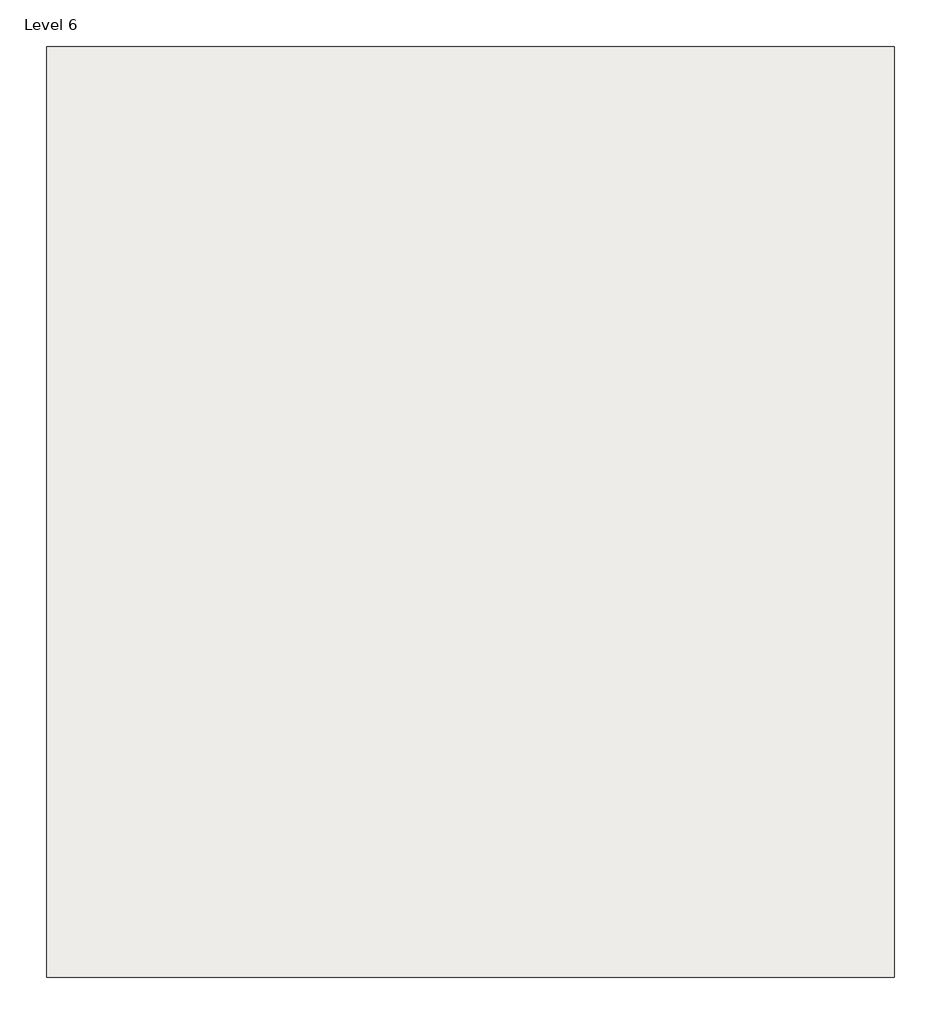
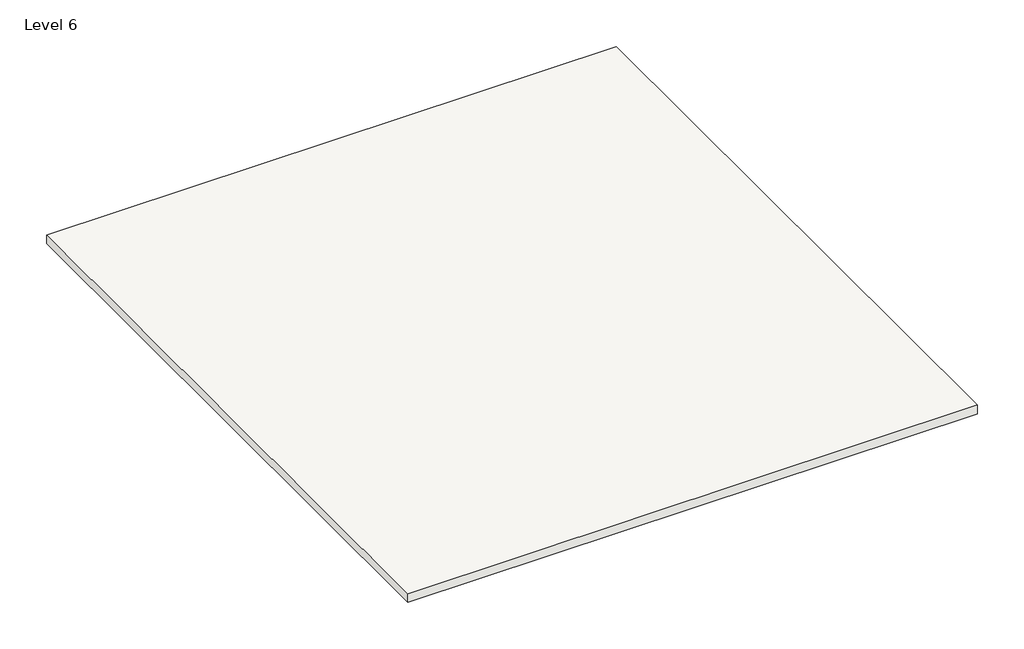
# One storey, incomplete: 1 roof.
"""IFC4 building model written with IfcOpenShell, lengths in millimetres."""

from ifc_helpers import new_model, si_unit, frame, origin, place, context, project, spatial, polyline, outline, extrude, element, save

model = new_model("IFC4")

# Units and contexts
model_context = context("Model", 3, world=origin())
ifc_project = project(units=[si_unit("LENGTHUNIT", "METRE", prefix="MILLI")], contexts=[model_context])

# Site, building, storey
site = spatial("IfcSite", under=ifc_project)
building = spatial("IfcBuilding", under=site)
storey = spatial("IfcBuildingStorey", under=building, Name="Level 6", Elevation=12801.6)

# Roof
placement = place(None, origin())
element("IfcRoof", 1, ObjectType="Generic - 12\"", at=placement, inside=storey, context=model_context, shape_type="SweptSolid", body=[
    extrude(outline(polyline([(-5539.1148498, 5385.7183073), (3909.6851502, 5385.7183073), (3909.6851502, -4993.3566927), (-5539.1148498, -4993.3566927), (-5539.1148498, 5385.7183073)])), frame((0.0, 0.0, 12649.2), z_axis=(0.0, 0.0, 1.0), x_axis=(1.0, 0.0, 0.0)), (0.0, 0.0, 1.0), 152.4),
])

save(model, "model.ifc")

# Revit data of these elements
# Type "Generic - 12\""
#   Assembly Code = "B1020"
#   Layers, outside or top first: 0' - 6" no material (function 1)
# Element 1 (IfcRoof, "Generic - 12\"")
#   built-in parameter 1001705 = 42 (stored number, unit not read)
#   built-in parameter 1001701 = -0.5 (stored number, unit not read)
#   built-in parameter 1001710 = 33615
#   Phase Created = New Construction
#   Materials on its faces: "Default Roof"
# Materials
#   "Default Roof": colour RGB 88 101 114, transparency 0, Cost = 0
